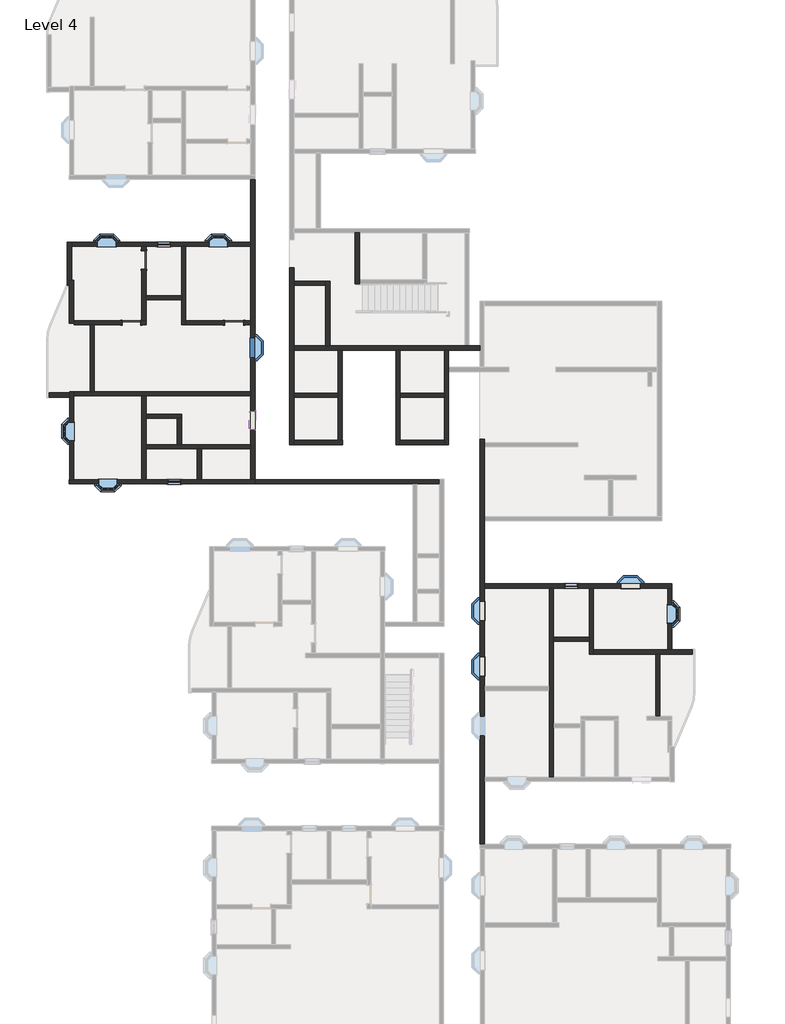
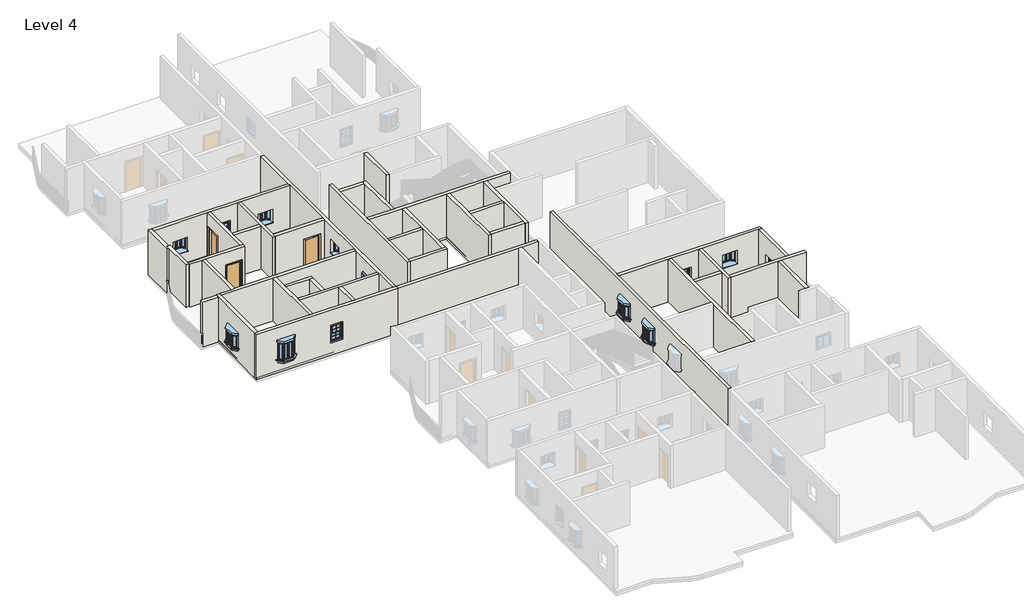
# One storey, part 3 of 14: 40 walls, 13 windows, 3 doors.
"""IFC4 building model written with IfcOpenShell, lengths in millimetres."""

from ifc_helpers import new_model, si_unit, frame, origin, place, context, project, spatial, polyline, outline, extrude, faceted_brep, transform, mapped, element, save
from components import door_54dd4da4, window_910x1210mm_154f9356, window_910x910mm_67ef725a, window_8debb0fa, windows_sgl_w_glazing_bars_910x910mm_256712d0

model = new_model("IFC4")

# Units and contexts
model_context = context("Model", 3, world=origin())
ifc_project = project(units=[si_unit("LENGTHUNIT", "METRE", prefix="MILLI")], contexts=[model_context])

# Site, building, storey
site = spatial("IfcSite", under=ifc_project)
building = spatial("IfcBuilding", under=site)
storey = spatial("IfcBuildingStorey", under=building, Name="Level 4", Elevation=9144.0)

# Doors
placement = place(None, origin())
door_shape = door_54dd4da4(model_context)
element("IfcDoor", 1, ObjectType="Single-Flush : 36\" x 84\"", at=placement, inside=storey, context=model_context, shape_type="MappedRepresentation", body=[
    mapped(door_shape, transform((-11210.3891351, 10605.7083494, 9144.0), x_axis=(1.0, 0.0, 0.0), y_axis=(0.0, 1.0, 0.0), z_axis=(0.0, 0.0, 1.0))),
])
element("IfcDoor", 2, ObjectType="Single-Flush : 36\" x 84\"", at=placement, inside=storey, context=model_context, shape_type="MappedRepresentation", body=[
    mapped(door_shape, transform((-15610.9391351, 13672.7583494, 9144.0), x_axis=(0.0, -1.0, 0.0), y_axis=(1.0, 0.0, 0.0), z_axis=(0.0, 0.0, 1.0))),
])
element("IfcDoor", 3, ObjectType="Single-Flush : 36\" x 84\"", at=placement, inside=storey, context=model_context, shape_type="MappedRepresentation", body=[
    mapped(door_shape, transform((-16220.5391351, 10605.7083494, 9144.0), x_axis=(1.0, 0.0, 0.0), y_axis=(0.0, 1.0, 0.0), z_axis=(0.0, 0.0, 1.0))),
])

# Walls
element("IfcWall", 4, ObjectType="4.5\" p", at=placement, inside=storey, context=model_context, shape_type="Brep", body=[
    faceted_brep([(-15509.3391351, 4456.3873146, 9144.0), (-13007.4391351, 4456.3873146, 9144.0), (-12804.2391351, 4456.3873146, 9144.0), (-10397.5891351, 4456.3873146, 9144.0), (-10397.5891351, 4456.3873146, 12192.0), (-12804.2391351, 4456.3873146, 12192.0), (-13007.4391351, 4456.3873146, 12192.0), (-15509.3391351, 4456.3873146, 12192.0), (-15509.3391351, 4659.5873146, 9144.0), (-15509.3391351, 4659.5873146, 12192.0), (-13985.3391351, 4659.5873146, 12192.0), (-13782.1391351, 4659.5873146, 12192.0), (-10397.5891351, 4659.5873146, 12192.0), (-10397.5891351, 4659.5873146, 9144.0), (-13782.1391351, 4659.5873146, 9144.0), (-13985.3391351, 4659.5873146, 9144.0)], [[[0, 1, 2, 3, 4, 5, 6, 7]], [[8, 9, 10, 11, 12, 13, 14, 15]], [[3, 2, 1, 0, 8, 15, 14, 13]], [[7, 6, 5, 4, 12, 11, 10, 9]], [[4, 3, 13, 12]], [[0, 7, 9, 8]]]),
])
element("IfcWall", 5, ObjectType="4.5\" p", at=placement, inside=storey, context=model_context, shape_type="SweptSolid", body=[
    extrude(outline(polyline([(-13007.4391351, 2953.9583494), (-13007.4391351, 4456.3873146), (-12804.2391351, 4456.3873146), (-12804.2391351, 2953.9583494), (-13007.4391351, 2953.9583494)])), frame((0.0, 0.0, 9144.0), z_axis=(0.0, 0.0, 1.0), x_axis=(1.0, 0.0, 0.0)), (0.0, 0.0, 1.0), 3048.0),
])
element("IfcWall", 6, ObjectType="4.5\" p", at=placement, inside=storey, context=model_context, shape_type="Brep", body=[
    faceted_brep([(-15509.3391351, 5953.2975261, 9144.0), (-13985.3391351, 5953.2975261, 9144.0), (-13782.1391351, 5953.2975261, 9144.0), (-13782.1391351, 5953.2975261, 12192.0), (-13985.3391351, 5953.2975261, 12192.0), (-15509.3391351, 5953.2975261, 12192.0), (-15509.3391351, 6156.4975261, 9144.0), (-15509.3391351, 6156.4975261, 12192.0), (-13782.1391351, 6156.4975261, 12192.0), (-13782.1391351, 6156.4975261, 9144.0)], [[[0, 1, 2, 3, 4, 5]], [[6, 7, 8, 9]], [[2, 1, 0, 6, 9]], [[5, 4, 3, 8, 7]], [[0, 5, 7, 6]], [[3, 2, 9, 8]]]),
])
element("IfcWall", 7, ObjectType="4.5\" p", at=placement, inside=storey, context=model_context, shape_type="SweptSolid", body=[
    extrude(outline(polyline([(-13985.3391351, 4659.5873146), (-13985.3391351, 5953.2975261), (-13782.1391351, 5953.2975261), (-13782.1391351, 4659.5873146), (-13985.3391351, 4659.5873146)])), frame((0.0, 0.0, 9144.0), z_axis=(0.0, 0.0, 1.0), x_axis=(1.0, 0.0, 0.0)), (0.0, 0.0, 1.0), 3048.0),
])
element("IfcWall", 8, ObjectType="4.5\" p", at=placement, inside=storey, context=model_context, shape_type="Brep", body=[
    faceted_brep([(-15712.5391351, 13215.5583494, 11277.6), (-15712.5391351, 13215.5583494, 9144.0), (-15712.5391351, 10707.3083494, 9144.0), (-15712.5391351, 10707.3083494, 12192.0), (-15712.5391351, 14333.1583494, 12192.0), (-15712.5391351, 14333.1583494, 9144.0), (-15712.5391351, 14129.9583494, 9144.0), (-15712.5391351, 14129.9583494, 11277.6), (-15509.3391351, 10707.3083494, 9144.0), (-15509.3391351, 11723.3083494, 9144.0), (-15509.3391351, 11926.5083494, 9144.0), (-15509.3391351, 13215.5583494, 9144.0), (-15509.3391351, 13215.5583494, 11277.6), (-15509.3391351, 14129.9583494, 11277.6), (-15509.3391351, 14129.9583494, 9144.0), (-15509.3391351, 14333.1583494, 9144.0), (-15509.3391351, 14333.1583494, 12192.0), (-15509.3391351, 11926.5083494, 12192.0), (-15509.3391351, 11723.3083494, 12192.0), (-15509.3391351, 10707.3083494, 12192.0)], [[[0, 1, 2, 3, 4, 5, 6, 7]], [[8, 9, 10, 11, 12, 13, 14, 15, 16, 17, 18, 19]], [[6, 5, 15, 14]], [[2, 1, 11, 10, 9, 8]], [[4, 3, 19, 18, 17, 16]], [[3, 2, 8, 19]], [[5, 4, 16, 15]], [[12, 11, 1, 0]], [[13, 12, 0, 7]], [[14, 13, 7, 6]]]),
])
element("IfcWall", 9, ObjectType="4.5\" p", at=placement, inside=storey, context=model_context, shape_type="Brep", body=[
    faceted_brep([(-13769.4391351, 14333.1583494, 9144.0), (-13769.4391351, 11926.5083494, 9144.0), (-13769.4391351, 11723.3083494, 9144.0), (-13769.4391351, 10504.1083494, 9144.0), (-13769.4391351, 10504.1083494, 12192.0), (-13769.4391351, 11723.3083494, 12192.0), (-13769.4391351, 11926.5083494, 12192.0), (-13769.4391351, 14333.1583494, 12192.0), (-13566.2391351, 14333.1583494, 9144.0), (-13566.2391351, 14333.1583494, 12192.0), (-13566.2391351, 10707.3083494, 12192.0), (-13566.2391351, 10504.1083494, 12192.0), (-13566.2391351, 10504.1083494, 9144.0), (-13566.2391351, 10707.3083494, 9144.0)], [[[0, 1, 2, 3, 4, 5, 6, 7]], [[8, 9, 10, 11, 12, 13]], [[3, 2, 1, 0, 8, 13, 12]], [[7, 6, 5, 4, 11, 10, 9]], [[0, 7, 9, 8]], [[4, 3, 12, 11]]]),
])
element("IfcWall", 10, ObjectType="4.5\" p", at=placement, inside=storey, context=model_context, shape_type="SweptSolid", body=[
    extrude(outline(polyline([(11277.6, -10753.1891351), (9144.0, -10753.1891351), (9144.0, -10397.5891351), (12192.0, -10397.5891351), (12192.0, -13566.2391351), (9144.0, -13566.2391351), (9144.0, -11667.5891351), (11277.6, -11667.5891351), (11277.6, -10753.1891351)])), frame((0.0, 10504.1083494, 0.0), z_axis=(0.0, 1.0, 0.0), x_axis=(0.0, 0.0, 1.0)), (0.0, 0.0, 1.0), 203.2),
])
element("IfcWall", 11, ObjectType="4.5\" p", at=placement, inside=storey, context=model_context, shape_type="SweptSolid", body=[
    extrude(outline(polyline([(-13769.4391351, 11723.3083494), (-15509.3391351, 11723.3083494), (-15509.3391351, 11926.5083494), (-13769.4391351, 11926.5083494), (-13769.4391351, 11723.3083494)])), frame((0.0, 0.0, 9144.0), z_axis=(0.0, 0.0, 1.0), x_axis=(1.0, 0.0, 0.0)), (0.0, 0.0, 1.0), 3048.0),
])
element("IfcWall", 12, ObjectType="4.5\" p", at=placement, inside=storey, context=model_context, shape_type="SweptSolid", body=[
    extrude(outline(polyline([(-6739.9891351, 12429.8715905), (-8289.3891351, 12429.8715905), (-8289.3891351, 12633.0715905), (-6739.9891351, 12633.0715905), (-6739.9891351, 12429.8715905)])), frame((0.0, 0.0, 9144.0), z_axis=(0.0, 0.0, 1.0), x_axis=(1.0, 0.0, 0.0)), (0.0, 0.0, 1.0), 3048.0),
])
element("IfcWall", 13, ObjectType="4.5\" p", at=placement, inside=storey, context=model_context, shape_type="SweptSolid", body=[
    extrude(outline(polyline([(-6130.3891351, 6970.2449943), (-8289.3891351, 6970.2449943), (-8289.3891351, 7173.4449943), (-6130.3891351, 7173.4449943), (-6130.3891351, 6970.2449943)])), frame((0.0, 0.0, 9144.0), z_axis=(0.0, 0.0, 1.0), x_axis=(1.0, 0.0, 0.0)), (0.0, 0.0, 1.0), 3048.0),
])
element("IfcWall", 14, ObjectType="4.5\" p", at=placement, inside=storey, context=model_context, shape_type="SweptSolid", body=[
    extrude(outline(polyline([(-948.7891351, 6970.2449943), (-3107.7891351, 6970.2449943), (-3107.7891351, 7173.4449943), (-948.7891351, 7173.4449943), (-948.7891351, 6970.2449943)])), frame((0.0, 0.0, 9144.0), z_axis=(0.0, 0.0, 1.0), x_axis=(1.0, 0.0, 0.0)), (0.0, 0.0, 1.0), 3048.0),
])
element("IfcWall", 15, ObjectType="4.5\" p", at=placement, inside=storey, context=model_context, shape_type="Brep", body=[
    faceted_brep([(-5298.5391351, 14988.9215905, 9144.0), (-5298.5391351, 12506.0715905, 9144.0), (-5298.5391351, 12506.0715905, 12192.0), (-5298.5391351, 14988.9215905, 12192.0), (-5095.3391351, 14988.9215905, 9144.0), (-5095.3391351, 14988.9215905, 12192.0), (-5095.3391351, 12709.2715905, 12192.0), (-5095.3391351, 12506.0715905, 12192.0), (-5095.3391351, 12506.0715905, 9144.0), (-5095.3391351, 12709.2715905, 9144.0)], [[[0, 1, 2, 3]], [[4, 5, 6, 7, 8, 9]], [[1, 0, 4, 9, 8]], [[3, 2, 7, 6, 5]], [[0, 3, 5, 4]], [[2, 1, 8, 7]]]),
])
element("IfcWall", 16, ObjectType="4.5\" p", at=placement, inside=storey, context=model_context, shape_type="SweptSolid", body=[
    extrude(outline(polyline([(-948.7891351, 4665.1949943), (-3107.7891351, 4665.1949943), (-3107.7891351, 4868.3949943), (-948.7891351, 4868.3949943), (-948.7891351, 4665.1949943)])), frame((0.0, 0.0, 9144.0), z_axis=(0.0, 0.0, 1.0), x_axis=(1.0, 0.0, 0.0)), (0.0, 0.0, 1.0), 3048.0),
])
element("IfcWall", 17, ObjectType="4.5\" p", at=placement, inside=storey, context=model_context, shape_type="Brep", body=[
    faceted_brep([(4184.4880523, -2336.4042694, 9144.0), (4184.4880523, -7130.6542694, 9144.0), (4184.4880523, -7333.8542694, 9144.0), (4184.4880523, -11556.6042694, 9144.0), (4184.4880523, -11556.6042694, 12192.0), (4184.4880523, -7333.8542694, 12192.0), (4184.4880523, -7130.6542694, 12192.0), (4184.4880523, -2336.4042694, 12192.0), (4387.6880523, -2336.4042694, 9144.0), (4387.6880523, -2336.4042694, 12192.0), (4387.6880523, -4736.7042694, 12192.0), (4387.6880523, -4939.9042694, 12192.0), (4387.6880523, -8959.4542694, 12192.0), (4387.6880523, -9162.6542694, 12192.0), (4387.6880523, -11556.6042694, 12192.0), (4387.6880523, -11556.6042694, 9144.0), (4387.6880523, -9162.6542694, 9144.0), (4387.6880523, -8959.4542694, 9144.0), (4387.6880523, -4939.9042694, 9144.0), (4387.6880523, -4736.7042694, 9144.0)], [[[0, 1, 2, 3, 4, 5, 6, 7]], [[8, 9, 10, 11, 12, 13, 14, 15, 16, 17, 18, 19]], [[3, 2, 1, 0, 8, 19, 18, 17, 16, 15]], [[7, 6, 5, 4, 14, 13, 12, 11, 10, 9]], [[4, 3, 15, 14]], [[0, 7, 9, 8]]]),
])
element("IfcWall", 18, ObjectType="4.5\" p", at=placement, inside=storey, context=model_context, shape_type="Brep", body=[
    faceted_brep([(803.8108649, 4915.2957306, 9144.0), (803.8108649, -14845.9042694, 9144.0), (803.8108649, -14845.9042694, 12192.0), (803.8108649, 4915.2957306, 12192.0), (803.8108649, -9516.0542694, 11254.0), (803.8108649, -9516.0542694, 10344.0), (803.8108649, -8606.0542694, 10344.0), (803.8108649, -8606.0542694, 11254.0), (803.8108649, -3909.0042694, 11254.0), (803.8108649, -3909.0042694, 10344.0), (803.8108649, -2999.0042694, 10344.0), (803.8108649, -2999.0042694, 11254.0), (803.8108649, -6620.4542694, 11254.0), (803.8108649, -6620.4542694, 10344.0), (803.8108649, -5710.4542694, 10344.0), (803.8108649, -5710.4542694, 11254.0), (1007.0108649, 4915.2957306, 9144.0), (1007.0108649, 4915.2957306, 12192.0), (1007.0108649, 4754.0949943, 12192.0), (1007.0108649, 4550.8949943, 12192.0), (1007.0108649, 1143.3957306, 12192.0), (1007.0108649, 940.1957306, 12192.0), (1007.0108649, -2133.2042694, 12192.0), (1007.0108649, -2336.4042694, 12192.0), (1007.0108649, -7130.6542694, 12192.0), (1007.0108649, -7333.8542694, 12192.0), (1007.0108649, -11556.6042694, 12192.0), (1007.0108649, -11759.8042694, 12192.0), (1007.0108649, -14845.9042694, 12192.0), (1007.0108649, -14845.9042694, 9144.0), (1007.0108649, -11759.8042694, 9144.0), (1007.0108649, -11556.6042694, 9144.0), (1007.0108649, -7333.8542694, 9144.0), (1007.0108649, -7130.6542694, 9144.0), (1007.0108649, -2336.4042694, 9144.0), (1007.0108649, -2133.2042694, 9144.0), (1007.0108649, 940.1957306, 9144.0), (1007.0108649, 1143.3957306, 9144.0), (1007.0108649, 4550.8949943, 9144.0), (1007.0108649, 4754.0949943, 9144.0), (1007.0108649, -9516.0542694, 11254.0), (1007.0108649, -8606.0542694, 11254.0), (1007.0108649, -8606.0542694, 10344.0), (1007.0108649, -9516.0542694, 10344.0), (1007.0108649, -3909.0042694, 11254.0), (1007.0108649, -2999.0042694, 11254.0), (1007.0108649, -2999.0042694, 10344.0), (1007.0108649, -3909.0042694, 10344.0), (1007.0108649, -6620.4542694, 11254.0), (1007.0108649, -5710.4542694, 11254.0), (1007.0108649, -5710.4542694, 10344.0), (1007.0108649, -6620.4542694, 10344.0)], [[[0, 1, 2, 3], [4, 5, 6, 7], [8, 9, 10, 11], [12, 13, 14, 15]], [[16, 17, 18, 19, 20, 21, 22, 23, 24, 25, 26, 27, 28, 29, 30, 31, 32, 33, 34, 35, 36, 37, 38, 39], [40, 41, 42, 43], [44, 45, 46, 47], [48, 49, 50, 51]], [[1, 0, 16, 39, 38, 37, 36, 35, 34, 33, 32, 31, 30, 29]], [[3, 2, 28, 27, 26, 25, 24, 23, 22, 21, 20, 19, 18, 17]], [[0, 3, 17, 16]], [[2, 1, 29, 28]], [[5, 4, 40, 43]], [[6, 5, 43, 42]], [[7, 6, 42, 41]], [[4, 7, 41, 40]], [[9, 8, 44, 47]], [[10, 9, 47, 46]], [[11, 10, 46, 45]], [[8, 11, 45, 44]], [[13, 12, 48, 51]], [[14, 13, 51, 50]], [[15, 14, 50, 49]], [[12, 15, 49, 48]]]),
])
element("IfcWall", 19, ObjectType="4.5\" p", at=placement, inside=storey, context=model_context, shape_type="SweptSolid", body=[
    extrude(outline(polyline([(6127.5880523, -4939.9042694), (4387.6880523, -4939.9042694), (4387.6880523, -4736.7042694), (6127.5880523, -4736.7042694), (6127.5880523, -4939.9042694)])), frame((0.0, 0.0, 9144.0), z_axis=(0.0, 0.0, 1.0), x_axis=(1.0, 0.0, 0.0)), (0.0, 0.0, 1.0), 3048.0),
])
element("IfcWall", 20, ObjectType="4.5\" p", at=placement, inside=storey, context=model_context, shape_type="Brep", body=[
    faceted_brep([(6127.5880523, -2336.4042694, 9144.0), (6127.5880523, -4736.7042694, 9144.0), (6127.5880523, -4939.9042694, 9144.0), (6127.5880523, -5555.8542694, 9144.0), (6127.5880523, -5555.8542694, 12192.0), (6127.5880523, -4939.9042694, 12192.0), (6127.5880523, -4736.7042694, 12192.0), (6127.5880523, -2336.4042694, 12192.0), (6330.7880523, -2336.4042694, 9144.0), (6330.7880523, -2336.4042694, 12192.0), (6330.7880523, -5352.6542694, 12192.0), (6330.7880523, -5555.8542694, 12192.0), (6330.7880523, -5555.8542694, 9144.0), (6330.7880523, -5352.6542694, 9144.0)], [[[0, 1, 2, 3, 4, 5, 6, 7]], [[8, 9, 10, 11, 12, 13]], [[3, 2, 1, 0, 8, 13, 12]], [[7, 6, 5, 4, 11, 10, 9]], [[0, 7, 9, 8]], [[4, 3, 12, 11]]]),
])
element("IfcWall", 21, ObjectType="4.5\" p", at=placement, inside=storey, context=model_context, shape_type="Brep", body=[
    faceted_brep([(6330.7880523, -5555.8542694, 9144.0), (9371.2322031, -5555.8542694, 9144.0), (9574.4322031, -5555.8542694, 9144.0), (11163.1380523, -5555.8542694, 9144.0), (11163.1380523, -5555.8542694, 12192.0), (9574.4322031, -5555.8542694, 12192.0), (9371.2322031, -5555.8542694, 12192.0), (6330.7880523, -5555.8542694, 12192.0), (6330.7880523, -5352.6542694, 9144.0), (6330.7880523, -5352.6542694, 12192.0), (9956.6380523, -5352.6542694, 12192.0), (10159.8380523, -5352.6542694, 12192.0), (11163.1380523, -5352.6542694, 12192.0), (11163.1380523, -5352.6542694, 9144.0), (10159.8380523, -5352.6542694, 9144.0), (9956.6380523, -5352.6542694, 9144.0)], [[[0, 1, 2, 3, 4, 5, 6, 7]], [[8, 9, 10, 11, 12, 13, 14, 15]], [[3, 2, 1, 0, 8, 15, 14, 13]], [[4, 3, 13, 12]], [[7, 6, 5, 4, 12, 11, 10, 9]], [[0, 7, 9, 8]]]),
])
element("IfcWall", 22, ObjectType="4.5\" p", at=placement, inside=storey, context=model_context, shape_type="SweptSolid", body=[
    extrude(outline(polyline([(9371.2322031, -8578.4542694), (9371.2322031, -5555.8542694), (9574.4322031, -5555.8542694), (9574.4322031, -8578.4542694), (9371.2322031, -8578.4542694)])), frame((0.0, 0.0, 9144.0), z_axis=(0.0, 0.0, 1.0), x_axis=(1.0, 0.0, 0.0)), (0.0, 0.0, 1.0), 3048.0),
])
element("IfcWall", 23, ObjectType="9\"", at=placement, inside=storey, context=model_context, shape_type="Brep", body=[
    faceted_brep([(-10181.6891351, 2953.9583494, 9144.0), (-10194.3891351, 2953.9583494, 9144.0), (-10397.5891351, 2953.9583494, 9144.0), (-12804.2391351, 2953.9583494, 9144.0), (-13007.4391351, 2953.9583494, 9144.0), (-15509.3391351, 2953.9583494, 9144.0), (-15712.5391351, 2953.9583494, 9144.0), (-19033.5891351, 2953.9583494, 9144.0), (-19236.7891351, 2953.9583494, 9144.0), (-19249.4891351, 2953.9583494, 9144.0), (-19249.4891351, 2953.9583494, 12192.0), (-19236.7891351, 2953.9583494, 12192.0), (-19033.5891351, 2953.9583494, 12192.0), (-15712.5391351, 2953.9583494, 12192.0), (-15509.3391351, 2953.9583494, 12192.0), (-13007.4391351, 2953.9583494, 12192.0), (-12804.2391351, 2953.9583494, 12192.0), (-10397.5891351, 2953.9583494, 12192.0), (-10194.3891351, 2953.9583494, 12192.0), (-10181.6891351, 2953.9583494, 12192.0), (-13794.8391351, 2953.9583494, 11125.2), (-14455.2391351, 2953.9583494, 11125.2), (-14455.2391351, 2953.9583494, 10058.4), (-13794.8391351, 2953.9583494, 10058.4), (-16918.0641351, 2953.9583494, 11268.4), (-17828.0641351, 2953.9583494, 11268.4), (-17828.0641351, 2953.9583494, 10058.4), (-16918.0641351, 2953.9583494, 10058.4), (-10181.6891351, 2750.7583494, 9144.0), (-10181.6891351, 2750.7583494, 12192.0), (-19249.4891351, 2750.7583494, 12192.0), (-19249.4891351, 2750.7583494, 9144.0), (-13794.8391351, 2750.7583494, 11125.2), (-13794.8391351, 2750.7583494, 10058.4), (-14455.2391351, 2750.7583494, 10058.4), (-14455.2391351, 2750.7583494, 11125.2), (-16918.0641351, 2750.7583494, 11268.4), (-16918.0641351, 2750.7583494, 10058.4), (-17828.0641351, 2750.7583494, 10058.4), (-17828.0641351, 2750.7583494, 11268.4)], [[[0, 1, 2, 3, 4, 5, 6, 7, 8, 9, 10, 11, 12, 13, 14, 15, 16, 17, 18, 19], [20, 21, 22, 23], [24, 25, 26, 27]], [[28, 29, 30, 31], [32, 33, 34, 35], [36, 37, 38, 39]], [[9, 8, 7, 6, 5, 4, 3, 2, 1, 0, 28, 31]], [[10, 9, 31, 30]], [[19, 18, 17, 16, 15, 14, 13, 12, 11, 10, 30, 29]], [[0, 19, 29, 28]], [[33, 32, 20, 23]], [[34, 33, 23, 22]], [[35, 34, 22, 21]], [[32, 35, 21, 20]], [[37, 36, 24, 27]], [[38, 37, 27, 26]], [[39, 38, 26, 25]], [[36, 39, 25, 24]]]),
])
element("IfcWall", 24, ObjectType="9\"", at=placement, inside=storey, context=model_context, shape_type="Brep", body=[
    faceted_brep([(-19033.5891351, 2953.9583494, 9144.0), (-19033.5891351, 7037.0083494, 9144.0), (-19033.5891351, 7240.2083494, 9144.0), (-19033.5891351, 7240.2083494, 12192.0), (-19033.5891351, 7037.0083494, 12192.0), (-19033.5891351, 2953.9583494, 12192.0), (-19033.5891351, 4854.8083494, 10968.4), (-19033.5891351, 5764.8083494, 10968.4), (-19033.5891351, 5764.8083494, 10058.4), (-19033.5891351, 4854.8083494, 10058.4), (-19236.7891351, 2953.9583494, 9144.0), (-19236.7891351, 2953.9583494, 12192.0), (-19236.7891351, 7240.2083494, 12192.0), (-19236.7891351, 7240.2083494, 9144.0), (-19236.7891351, 4854.8083494, 10968.4), (-19236.7891351, 4854.8083494, 10058.4), (-19236.7891351, 5764.8083494, 10058.4), (-19236.7891351, 5764.8083494, 10968.4)], [[[0, 1, 2, 3, 4, 5], [6, 7, 8, 9]], [[10, 11, 12, 13], [14, 15, 16, 17]], [[2, 1, 0, 10, 13]], [[5, 4, 3, 12, 11]], [[0, 5, 11, 10]], [[3, 2, 13, 12]], [[15, 14, 6, 9]], [[16, 15, 9, 8]], [[17, 16, 8, 7]], [[14, 17, 7, 6]]]),
])
element("IfcWall", 25, ObjectType="9\"", at=placement, inside=storey, context=model_context, shape_type="Brep", body=[
    faceted_brep([(-10194.3891351, 2953.9583494, 9144.0), (-10194.3891351, 17597.0583494, 9144.0), (-10194.3891351, 17597.0583494, 12192.0), (-10194.3891351, 2953.9583494, 12192.0), (-10194.3891351, 9841.5083494, 11254.0), (-10194.3891351, 9841.5083494, 10344.0), (-10194.3891351, 8931.5083494, 10344.0), (-10194.3891351, 8931.5083494, 11254.0), (-10194.3891351, 5393.297832, 11254.0), (-10194.3891351, 6303.297832, 11254.0), (-10194.3891351, 6303.297832, 10344.0), (-10194.3891351, 5393.297832, 10344.0), (-10397.5891351, 2953.9583494, 9144.0), (-10397.5891351, 2953.9583494, 12192.0), (-10397.5891351, 4456.3873146, 12192.0), (-10397.5891351, 4659.5873146, 12192.0), (-10397.5891351, 7037.0083494, 12192.0), (-10397.5891351, 7240.2083494, 12192.0), (-10397.5891351, 10504.1083494, 12192.0), (-10397.5891351, 10707.3083494, 12192.0), (-10397.5891351, 14333.1583494, 12192.0), (-10397.5891351, 14536.3583494, 12192.0), (-10397.5891351, 17597.0583494, 12192.0), (-10397.5891351, 17597.0583494, 9144.0), (-10397.5891351, 14536.3583494, 9144.0), (-10397.5891351, 14333.1583494, 9144.0), (-10397.5891351, 10707.3083494, 9144.0), (-10397.5891351, 10504.1083494, 9144.0), (-10397.5891351, 7240.2083494, 9144.0), (-10397.5891351, 7037.0083494, 9144.0), (-10397.5891351, 4659.5873146, 9144.0), (-10397.5891351, 4456.3873146, 9144.0), (-10397.5891351, 9841.5083494, 11254.0), (-10397.5891351, 8931.5083494, 11254.0), (-10397.5891351, 8931.5083494, 10344.0), (-10397.5891351, 9841.5083494, 10344.0), (-10397.5891351, 5393.297832, 11254.0), (-10397.5891351, 5393.297832, 10344.0), (-10397.5891351, 6303.297832, 10344.0), (-10397.5891351, 6303.297832, 11254.0)], [[[0, 1, 2, 3], [4, 5, 6, 7], [8, 9, 10, 11]], [[12, 13, 14, 15, 16, 17, 18, 19, 20, 21, 22, 23, 24, 25, 26, 27, 28, 29, 30, 31], [32, 33, 34, 35], [36, 37, 38, 39]], [[1, 0, 12, 31, 30, 29, 28, 27, 26, 25, 24, 23]], [[2, 1, 23, 22]], [[3, 2, 22, 21, 20, 19, 18, 17, 16, 15, 14, 13]], [[0, 3, 13, 12]], [[5, 4, 32, 35]], [[6, 5, 35, 34]], [[7, 6, 34, 33]], [[4, 7, 33, 32]], [[37, 36, 8, 11]], [[38, 37, 11, 10]], [[39, 38, 10, 9]], [[36, 39, 9, 8]]]),
])
element("IfcWall", 26, ObjectType="9\"", at=placement, inside=storey, context=model_context, shape_type="SweptSolid", body=[
    extrude(outline(polyline([(-19249.4891351, 6979.8583494), (-20240.0891351, 6979.8583494), (-20240.0891351, 7183.0583494), (-19249.4891351, 7183.0583494), (-19249.4891351, 6979.8583494)])), frame((0.0, 0.0, 9144.0), z_axis=(0.0, 0.0, 1.0), x_axis=(1.0, 0.0, 0.0)), (0.0, 0.0, 1.0), 3048.0),
])
element("IfcWall", 27, ObjectType="9\"", at=placement, inside=storey, context=model_context, shape_type="Brep", body=[
    faceted_brep([(-19147.8891351, 12435.1858981, 9144.0), (-19147.8891351, 14333.1583494, 9144.0), (-19147.8891351, 14536.3583494, 9144.0), (-19147.8891351, 14549.0583494, 9144.0), (-19147.8891351, 14549.0583494, 12192.0), (-19147.8891351, 14536.3583494, 12192.0), (-19147.8891351, 14333.1583494, 12192.0), (-19147.8891351, 12435.1858981, 12192.0), (-19351.0891351, 12435.1858981, 9144.0), (-19351.0891351, 12435.1858981, 12192.0), (-19351.0891351, 14549.0583494, 12192.0), (-19351.0891351, 14549.0583494, 9144.0)], [[[0, 1, 2, 3, 4, 5, 6, 7]], [[8, 9, 10, 11]], [[3, 2, 1, 0, 8, 11]], [[4, 3, 11, 10]], [[7, 6, 5, 4, 10, 9]], [[0, 7, 9, 8]]]),
])
element("IfcWall", 28, ObjectType="9\"", at=placement, inside=storey, context=model_context, shape_type="Brep", body=[
    faceted_brep([(-19147.8891351, 14333.1583494, 9144.0), (-15712.5391351, 14333.1583494, 9144.0), (-15509.3391351, 14333.1583494, 9144.0), (-13769.4391351, 14333.1583494, 9144.0), (-13566.2391351, 14333.1583494, 9144.0), (-10397.5891351, 14333.1583494, 9144.0), (-10397.5891351, 14333.1583494, 12192.0), (-13566.2391351, 14333.1583494, 12192.0), (-13769.4391351, 14333.1583494, 12192.0), (-15509.3391351, 14333.1583494, 12192.0), (-15712.5391351, 14333.1583494, 12192.0), (-19147.8891351, 14333.1583494, 12192.0), (-17885.2141351, 14333.1583494, 10968.4), (-16975.2141351, 14333.1583494, 10968.4), (-16975.2141351, 14333.1583494, 10058.4), (-17885.2141351, 14333.1583494, 10058.4), (-12436.9141351, 14333.1583494, 10968.4), (-11526.9141351, 14333.1583494, 10968.4), (-11526.9141351, 14333.1583494, 10058.4), (-12436.9141351, 14333.1583494, 10058.4), (-14309.1891351, 14333.1583494, 11125.2), (-14309.1891351, 14333.1583494, 10058.4), (-14969.5891351, 14333.1583494, 10058.4), (-14969.5891351, 14333.1583494, 11125.2), (-19147.8891351, 14536.3583494, 9144.0), (-19147.8891351, 14536.3583494, 12192.0), (-10397.5891351, 14536.3583494, 12192.0), (-10397.5891351, 14536.3583494, 9144.0), (-17885.2141351, 14536.3583494, 10968.4), (-17885.2141351, 14536.3583494, 10058.4), (-16975.2141351, 14536.3583494, 10058.4), (-16975.2141351, 14536.3583494, 10968.4), (-12436.9141351, 14536.3583494, 10968.4), (-12436.9141351, 14536.3583494, 10058.4), (-11526.9141351, 14536.3583494, 10058.4), (-11526.9141351, 14536.3583494, 10968.4), (-14309.1891351, 14536.3583494, 11125.2), (-14969.5891351, 14536.3583494, 11125.2), (-14969.5891351, 14536.3583494, 10058.4), (-14309.1891351, 14536.3583494, 10058.4)], [[[0, 1, 2, 3, 4, 5, 6, 7, 8, 9, 10, 11], [12, 13, 14, 15], [16, 17, 18, 19], [20, 21, 22, 23]], [[24, 25, 26, 27], [28, 29, 30, 31], [32, 33, 34, 35], [36, 37, 38, 39]], [[5, 4, 3, 2, 1, 0, 24, 27]], [[11, 10, 9, 8, 7, 6, 26, 25]], [[6, 5, 27, 26]], [[0, 11, 25, 24]], [[29, 28, 12, 15]], [[30, 29, 15, 14]], [[31, 30, 14, 13]], [[28, 31, 13, 12]], [[33, 32, 16, 19]], [[34, 33, 19, 18]], [[35, 34, 18, 17]], [[32, 35, 17, 16]], [[21, 20, 36, 39]], [[22, 21, 39, 38]], [[23, 22, 38, 37]], [[20, 23, 37, 36]]]),
])
element("IfcWall", 29, ObjectType="9\"", at=placement, inside=storey, context=model_context, shape_type="SweptSolid", body=[
    extrude(outline(polyline([(-19249.4891351, 10585.5474528), (-19249.4891351, 12672.4473407), (-19046.2891351, 12672.4473407), (-19046.2891351, 10585.5474528), (-19249.4891351, 10585.5474528)])), frame((0.0, 0.0, 9144.0), z_axis=(0.0, 0.0, 1.0), x_axis=(1.0, 0.0, 0.0)), (0.0, 0.0, 1.0), 3048.0),
])
element("IfcWall", 30, ObjectType="9\" w", at=placement, inside=storey, context=model_context, shape_type="Brep", body=[
    faceted_brep([(-1177.3891351, 2953.9583494, 9144.0), (-10181.6891351, 2953.9583494, 9144.0), (-10181.6891351, 2953.9583494, 12192.0), (-1177.3891351, 2953.9583494, 12192.0), (-1177.3891351, 2750.7583494, 9144.0), (-1177.3891351, 2750.7583494, 12192.0), (-2269.5891351, 2750.7583494, 12192.0), (-2472.7891351, 2750.7583494, 12192.0), (-10181.6891351, 2750.7583494, 12192.0), (-10181.6891351, 2750.7583494, 9144.0), (-2472.7891351, 2750.7583494, 9144.0), (-2269.5891351, 2750.7583494, 9144.0)], [[[0, 1, 2, 3]], [[4, 5, 6, 7, 8, 9, 10, 11]], [[1, 0, 4, 11, 10, 9]], [[2, 1, 9, 8]], [[3, 2, 8, 7, 6, 5]], [[0, 3, 5, 4]]]),
])
element("IfcWall", 31, ObjectType="9\" w", at=placement, inside=storey, context=model_context, shape_type="Brep", body=[
    faceted_brep([(-15763.3391351, 10504.1083494, 11277.6), (-15763.3391351, 10504.1083494, 9144.0), (-15509.3391351, 10504.1083494, 9144.0), (-15509.3391351, 10504.1083494, 12192.0), (-18042.9891351, 10504.1083494, 12192.0), (-18246.1891351, 10504.1083494, 12192.0), (-19027.2391351, 10504.1083494, 12192.0), (-19027.2391351, 10504.1083494, 9144.0), (-18246.1891351, 10504.1083494, 9144.0), (-18042.9891351, 10504.1083494, 9144.0), (-16677.7391351, 10504.1083494, 9144.0), (-16677.7391351, 10504.1083494, 11277.6), (-15509.3391351, 10707.3083494, 9144.0), (-15712.5391351, 10707.3083494, 9144.0), (-15763.3391351, 10707.3083494, 9144.0), (-15763.3391351, 10707.3083494, 11277.6), (-16677.7391351, 10707.3083494, 11277.6), (-16677.7391351, 10707.3083494, 9144.0), (-19027.2391351, 10707.3083494, 9144.0), (-19027.2391351, 10707.3083494, 12192.0), (-15712.5391351, 10707.3083494, 12192.0), (-15509.3391351, 10707.3083494, 12192.0)], [[[0, 1, 2, 3, 4, 5, 6, 7, 8, 9, 10, 11]], [[12, 13, 14, 15, 16, 17, 18, 19, 20, 21]], [[2, 1, 14, 13, 12]], [[10, 9, 8, 7, 18, 17]], [[6, 5, 4, 3, 21, 20, 19]], [[7, 6, 19, 18]], [[3, 2, 12, 21]], [[15, 14, 1, 0]], [[16, 15, 0, 11]], [[17, 16, 11, 10]]]),
])
element("IfcWall", 32, ObjectType="9\" w", at=placement, inside=storey, context=model_context, shape_type="SweptSolid", body=[
    extrude(outline(polyline([(-18246.1891351, 7240.2083494), (-18246.1891351, 10504.1083494), (-18042.9891351, 10504.1083494), (-18042.9891351, 7240.2083494), (-18246.1891351, 7240.2083494)])), frame((0.0, 0.0, 9144.0), z_axis=(0.0, 0.0, 1.0), x_axis=(1.0, 0.0, 0.0)), (0.0, 0.0, 1.0), 3048.0),
])
element("IfcWall", 33, ObjectType="9\" w", at=placement, inside=storey, context=model_context, shape_type="Brep", body=[
    faceted_brep([(-19033.5891351, 7037.0083494, 9144.0), (-15712.5391351, 7037.0083494, 9144.0), (-15509.3391351, 7037.0083494, 9144.0), (-10397.5891351, 7037.0083494, 9144.0), (-10397.5891351, 7037.0083494, 12192.0), (-15509.3391351, 7037.0083494, 12192.0), (-15712.5391351, 7037.0083494, 12192.0), (-19033.5891351, 7037.0083494, 12192.0), (-19033.5891351, 7240.2083494, 9144.0), (-19033.5891351, 7240.2083494, 12192.0), (-18246.1891351, 7240.2083494, 12192.0), (-18042.9891351, 7240.2083494, 12192.0), (-10397.5891351, 7240.2083494, 12192.0), (-10397.5891351, 7240.2083494, 9144.0), (-18042.9891351, 7240.2083494, 9144.0), (-18246.1891351, 7240.2083494, 9144.0)], [[[0, 1, 2, 3, 4, 5, 6, 7]], [[8, 9, 10, 11, 12, 13, 14, 15]], [[3, 2, 1, 0, 8, 15, 14, 13]], [[7, 6, 5, 4, 12, 11, 10, 9]], [[0, 7, 9, 8]], [[4, 3, 13, 12]]]),
])
element("IfcWall", 34, ObjectType="9\" w", at=placement, inside=storey, context=model_context, shape_type="Brep", body=[
    faceted_brep([(-15712.5391351, 7037.0083494, 9144.0), (-15712.5391351, 2953.9583494, 9144.0), (-15712.5391351, 2953.9583494, 12192.0), (-15712.5391351, 7037.0083494, 12192.0), (-15509.3391351, 7037.0083494, 9144.0), (-15509.3391351, 7037.0083494, 12192.0), (-15509.3391351, 6156.4975261, 12192.0), (-15509.3391351, 5953.2975261, 12192.0), (-15509.3391351, 4659.5873146, 12192.0), (-15509.3391351, 4456.3873146, 12192.0), (-15509.3391351, 2953.9583494, 12192.0), (-15509.3391351, 2953.9583494, 9144.0), (-15509.3391351, 4456.3873146, 9144.0), (-15509.3391351, 4659.5873146, 9144.0), (-15509.3391351, 5953.2975261, 9144.0), (-15509.3391351, 6156.4975261, 9144.0)], [[[0, 1, 2, 3]], [[4, 5, 6, 7, 8, 9, 10, 11, 12, 13, 14, 15]], [[1, 0, 4, 15, 14, 13, 12, 11]], [[3, 2, 10, 9, 8, 7, 6, 5]], [[2, 1, 11, 10]], [[0, 3, 5, 4]]]),
])
element("IfcWall", 35, ObjectType="9\" w", at=placement, inside=storey, context=model_context, shape_type="Brep", body=[
    faceted_brep([(-8492.5891351, 13295.1410318, 9144.0), (-8492.5891351, 4652.4949943, 9144.0), (-8492.5891351, 4652.4949943, 12192.0), (-8492.5891351, 13295.1410318, 12192.0), (-8289.3891351, 13295.1410318, 9144.0), (-8289.3891351, 13295.1410318, 12192.0), (-8289.3891351, 12633.0715905, 12192.0), (-8289.3891351, 12429.8715905, 12192.0), (-8289.3891351, 9478.4949943, 12192.0), (-8289.3891351, 9275.2949943, 12192.0), (-8289.3891351, 7173.4449943, 12192.0), (-8289.3891351, 6970.2449943, 12192.0), (-8289.3891351, 4868.3949943, 12192.0), (-8289.3891351, 4665.1949943, 12192.0), (-8289.3891351, 4652.4949943, 12192.0), (-8289.3891351, 4652.4949943, 9144.0), (-8289.3891351, 4665.1949943, 9144.0), (-8289.3891351, 4868.3949943, 9144.0), (-8289.3891351, 6970.2449943, 9144.0), (-8289.3891351, 7173.4449943, 9144.0), (-8289.3891351, 9275.2949943, 9144.0), (-8289.3891351, 9478.4949943, 9144.0), (-8289.3891351, 12429.8715905, 9144.0), (-8289.3891351, 12633.0715905, 9144.0)], [[[0, 1, 2, 3]], [[4, 5, 6, 7, 8, 9, 10, 11, 12, 13, 14, 15, 16, 17, 18, 19, 20, 21, 22, 23]], [[1, 0, 4, 23, 22, 21, 20, 19, 18, 17, 16, 15]], [[2, 1, 15, 14]], [[3, 2, 14, 13, 12, 11, 10, 9, 8, 7, 6, 5]], [[0, 3, 5, 4]]]),
])
element("IfcWall", 36, ObjectType="9\" w", at=placement, inside=storey, context=model_context, shape_type="Brep", body=[
    faceted_brep([(-8289.3891351, 4665.1949943, 9144.0), (-5914.4891351, 4665.1949943, 9144.0), (-5914.4891351, 4665.1949943, 12192.0), (-8289.3891351, 4665.1949943, 12192.0), (-8289.3891351, 4868.3949943, 9144.0), (-8289.3891351, 4868.3949943, 12192.0), (-6130.3891351, 4868.3949943, 12192.0), (-5927.1891351, 4868.3949943, 12192.0), (-5914.4891351, 4868.3949943, 12192.0), (-5914.4891351, 4868.3949943, 9144.0), (-5927.1891351, 4868.3949943, 9144.0), (-6130.3891351, 4868.3949943, 9144.0)], [[[0, 1, 2, 3]], [[4, 5, 6, 7, 8, 9, 10, 11]], [[1, 0, 4, 11, 10, 9]], [[2, 1, 9, 8]], [[3, 2, 8, 7, 6, 5]], [[0, 3, 5, 4]]]),
])
element("IfcWall", 37, ObjectType="9\" w", at=placement, inside=storey, context=model_context, shape_type="Brep", body=[
    faceted_brep([(-5927.1891351, 4868.3949943, 9144.0), (-5927.1891351, 9275.2949943, 9144.0), (-5927.1891351, 9275.2949943, 12192.0), (-5927.1891351, 4868.3949943, 12192.0), (-6130.3891351, 4868.3949943, 9144.0), (-6130.3891351, 4868.3949943, 12192.0), (-6130.3891351, 6970.2449943, 12192.0), (-6130.3891351, 7173.4449943, 12192.0), (-6130.3891351, 9275.2949943, 12192.0), (-6130.3891351, 9275.2949943, 9144.0), (-6130.3891351, 7173.4449943, 9144.0), (-6130.3891351, 6970.2449943, 9144.0)], [[[0, 1, 2, 3]], [[4, 5, 6, 7, 8, 9, 10, 11]], [[1, 0, 4, 11, 10, 9]], [[3, 2, 8, 7, 6, 5]], [[0, 3, 5, 4]], [[2, 1, 9, 8]]]),
])
element("IfcWall", 38, ObjectType="9\" w", at=placement, inside=storey, context=model_context, shape_type="Brep", body=[
    faceted_brep([(-8289.3891351, 9275.2949943, 9144.0), (-6130.3891351, 9275.2949943, 9144.0), (-5927.1891351, 9275.2949943, 9144.0), (-3310.9891351, 9275.2949943, 9144.0), (-3107.7891351, 9275.2949943, 9144.0), (-948.7891351, 9275.2949943, 9144.0), (-745.5891351, 9275.2949943, 9144.0), (793.5880523, 9275.2949943, 9144.0), (793.5880523, 9275.2949943, 12192.0), (-745.5891351, 9275.2949943, 12192.0), (-948.7891351, 9275.2949943, 12192.0), (-3107.7891351, 9275.2949943, 12192.0), (-3310.9891351, 9275.2949943, 12192.0), (-5927.1891351, 9275.2949943, 12192.0), (-6130.3891351, 9275.2949943, 12192.0), (-8289.3891351, 9275.2949943, 12192.0), (-8289.3891351, 9478.4949943, 9144.0), (-8289.3891351, 9478.4949943, 12192.0), (-6739.9891351, 9478.4949943, 12192.0), (-6536.7891351, 9478.4949943, 12192.0), (54.5108649, 9478.4949943, 12192.0), (257.7108649, 9478.4949943, 12192.0), (793.5880523, 9478.4949943, 12192.0), (793.5880523, 9478.4949943, 9144.0), (257.7108649, 9478.4949943, 9144.0), (54.5108649, 9478.4949943, 9144.0), (-6536.7891351, 9478.4949943, 9144.0), (-6739.9891351, 9478.4949943, 9144.0)], [[[0, 1, 2, 3, 4, 5, 6, 7, 8, 9, 10, 11, 12, 13, 14, 15]], [[16, 17, 18, 19, 20, 21, 22, 23, 24, 25, 26, 27]], [[7, 6, 5, 4, 3, 2, 1, 0, 16, 27, 26, 25, 24, 23]], [[15, 14, 13, 12, 11, 10, 9, 8, 22, 21, 20, 19, 18, 17]], [[0, 15, 17, 16]], [[8, 7, 23, 22]]]),
])
element("IfcWall", 39, ObjectType="9\" w", at=placement, inside=storey, context=model_context, shape_type="Brep", body=[
    faceted_brep([(-3310.9891351, 9275.2949943, 9144.0), (-3310.9891351, 4652.4949943, 9144.0), (-3310.9891351, 4652.4949943, 12192.0), (-3310.9891351, 9275.2949943, 12192.0), (-3107.7891351, 9275.2949943, 9144.0), (-3107.7891351, 9275.2949943, 12192.0), (-3107.7891351, 7173.4449943, 12192.0), (-3107.7891351, 6970.2449943, 12192.0), (-3107.7891351, 4868.3949943, 12192.0), (-3107.7891351, 4665.1949943, 12192.0), (-3107.7891351, 4652.4949943, 12192.0), (-3107.7891351, 4652.4949943, 9144.0), (-3107.7891351, 4665.1949943, 9144.0), (-3107.7891351, 4868.3949943, 9144.0), (-3107.7891351, 6970.2449943, 9144.0), (-3107.7891351, 7173.4449943, 9144.0)], [[[0, 1, 2, 3]], [[4, 5, 6, 7, 8, 9, 10, 11, 12, 13, 14, 15]], [[1, 0, 4, 15, 14, 13, 12, 11]], [[2, 1, 11, 10]], [[3, 2, 10, 9, 8, 7, 6, 5]], [[0, 3, 5, 4]]]),
])
element("IfcWall", 40, ObjectType="9\" w", at=placement, inside=storey, context=model_context, shape_type="Brep", body=[
    faceted_brep([(-745.5891351, 4652.4949943, 9144.0), (-745.5891351, 8223.6457306, 9144.0), (-745.5891351, 8426.8457306, 9144.0), (-745.5891351, 9275.2949943, 9144.0), (-745.5891351, 9275.2949943, 12192.0), (-745.5891351, 8426.8457306, 12192.0), (-745.5891351, 8223.6457306, 12192.0), (-745.5891351, 4652.4949943, 12192.0), (-948.7891351, 4652.4949943, 9144.0), (-948.7891351, 4652.4949943, 12192.0), (-948.7891351, 4665.1949943, 12192.0), (-948.7891351, 4868.3949943, 12192.0), (-948.7891351, 6970.2449943, 12192.0), (-948.7891351, 7173.4449943, 12192.0), (-948.7891351, 9275.2949943, 12192.0), (-948.7891351, 9275.2949943, 9144.0), (-948.7891351, 7173.4449943, 9144.0), (-948.7891351, 6970.2449943, 9144.0), (-948.7891351, 4868.3949943, 9144.0), (-948.7891351, 4665.1949943, 9144.0)], [[[0, 1, 2, 3, 4, 5, 6, 7]], [[8, 9, 10, 11, 12, 13, 14, 15, 16, 17, 18, 19]], [[3, 2, 1, 0, 8, 19, 18, 17, 16, 15]], [[7, 6, 5, 4, 14, 13, 12, 11, 10, 9]], [[0, 7, 9, 8]], [[4, 3, 15, 14]]]),
])
element("IfcWall", 41, ObjectType="9\" w", at=placement, inside=storey, context=model_context, shape_type="Brep", body=[
    faceted_brep([(-6536.7891351, 9478.4949943, 9144.0), (-6536.7891351, 12633.0715905, 9144.0), (-6536.7891351, 12633.0715905, 12192.0), (-6536.7891351, 9478.4949943, 12192.0), (-6739.9891351, 9478.4949943, 9144.0), (-6739.9891351, 9478.4949943, 12192.0), (-6739.9891351, 12429.8715905, 12192.0), (-6739.9891351, 12633.0715905, 12192.0), (-6739.9891351, 12633.0715905, 9144.0), (-6739.9891351, 12429.8715905, 9144.0)], [[[0, 1, 2, 3]], [[4, 5, 6, 7, 8, 9]], [[1, 0, 4, 9, 8]], [[3, 2, 7, 6, 5]], [[0, 3, 5, 4]], [[2, 1, 8, 7]]]),
])
element("IfcWall", 42, ObjectType="9\" w", at=placement, inside=storey, context=model_context, shape_type="Brep", body=[
    faceted_brep([(1007.0108649, -2336.4042694, 9144.0), (4184.4880523, -2336.4042694, 9144.0), (4387.6880523, -2336.4042694, 9144.0), (6127.5880523, -2336.4042694, 9144.0), (6330.7880523, -2336.4042694, 9144.0), (9956.6380523, -2336.4042694, 9144.0), (10159.8380523, -2336.4042694, 9144.0), (10172.5380523, -2336.4042694, 9144.0), (10172.5380523, -2336.4042694, 12192.0), (10159.8380523, -2336.4042694, 12192.0), (9956.6380523, -2336.4042694, 12192.0), (6330.7880523, -2336.4042694, 12192.0), (6127.5880523, -2336.4042694, 12192.0), (4387.6880523, -2336.4042694, 12192.0), (4184.4880523, -2336.4042694, 12192.0), (1007.0108649, -2336.4042694, 12192.0), (7688.7130523, -2336.4042694, 11254.0), (8598.7130523, -2336.4042694, 11254.0), (8598.7130523, -2336.4042694, 10344.0), (7688.7130523, -2336.4042694, 10344.0), (4927.4380523, -2336.4042694, 11125.2), (5587.8380523, -2336.4042694, 11125.2), (5587.8380523, -2336.4042694, 10058.4), (4927.4380523, -2336.4042694, 10058.4), (1007.0108649, -2133.2042694, 9144.0), (1007.0108649, -2133.2042694, 12192.0), (10172.5380523, -2133.2042694, 12192.0), (10172.5380523, -2133.2042694, 9144.0), (7688.7130523, -2133.2042694, 11254.0), (7688.7130523, -2133.2042694, 10344.0), (8598.7130523, -2133.2042694, 10344.0), (8598.7130523, -2133.2042694, 11254.0), (4927.4380523, -2133.2042694, 11125.2), (4927.4380523, -2133.2042694, 10058.4), (5587.8380523, -2133.2042694, 10058.4), (5587.8380523, -2133.2042694, 11125.2)], [[[0, 1, 2, 3, 4, 5, 6, 7, 8, 9, 10, 11, 12, 13, 14, 15], [16, 17, 18, 19], [20, 21, 22, 23]], [[24, 25, 26, 27], [28, 29, 30, 31], [32, 33, 34, 35]], [[7, 6, 5, 4, 3, 2, 1, 0, 24, 27]], [[8, 7, 27, 26]], [[15, 14, 13, 12, 11, 10, 9, 8, 26, 25]], [[0, 15, 25, 24]], [[29, 28, 16, 19]], [[30, 29, 19, 18]], [[31, 30, 18, 17]], [[28, 31, 17, 16]], [[33, 32, 20, 23]], [[34, 33, 23, 22]], [[35, 34, 22, 21]], [[32, 35, 21, 20]]]),
])
element("IfcWall", 43, ObjectType="9\" w", at=placement, inside=storey, context=model_context, shape_type="SweptSolid", body=[
    extrude(outline(polyline([(-2336.4042694, 9144.0), (-5352.6542694, 9144.0), (-5352.6542694, 12192.0), (-2336.4042694, 12192.0), (-2336.4042694, 9144.0)]), holes=[polyline([(-3151.4042694, 10968.4), (-4061.4042694, 10968.4), (-4061.4042694, 10058.4), (-3151.4042694, 10058.4), (-3151.4042694, 10968.4)])]), frame((9956.6380523, 0.0, 0.0), z_axis=(1.0, 0.0, 0.0), x_axis=(0.0, 1.0, 0.0)), (0.0, 0.0, 1.0), 203.2),
])

# Windows
window_910x1210mm_shape = window_910x1210mm_154f9356(model_context)
element("IfcWindow", 44, ObjectType="910x1210mm", at=placement, inside=storey, context=model_context, shape_type="MappedRepresentation", body=[
    mapped(window_910x1210mm_shape, transform((-17943.0641351, 2860.8149172, 9158.4), x_axis=(-1.0, 0.0, 0.0), y_axis=(0.0, -1.0, 0.0), z_axis=(0.0, 0.0, 1.0))),
])
window_910x910mm_shape = window_910x910mm_67ef725a(model_context)
element("IfcWindow", 45, ObjectType="910x910mm", at=placement, inside=storey, context=model_context, shape_type="MappedRepresentation", body=[
    mapped(window_910x910mm_shape, transform((8713.7130523, -2243.2608372, 9144.0), x_axis=(1.0, 0.0, 0.0), y_axis=(0.0, 1.0, 0.0), z_axis=(0.0, 0.0, 1.0))),
])
element("IfcWindow", 46, ObjectType="910x910mm", at=placement, inside=storey, context=model_context, shape_type="MappedRepresentation", body=[
    mapped(window_910x910mm_shape, transform((10049.7814845, -4176.4042694, 8858.4), x_axis=(0.0, -1.0, 0.0), y_axis=(1.0, 0.0, 0.0), z_axis=(0.0, 0.0, 1.0))),
])
element("IfcWindow", 47, ObjectType="910x910mm", at=placement, inside=storey, context=model_context, shape_type="MappedRepresentation", body=[
    mapped(window_910x910mm_shape, transform((-16860.2141351, 14426.3017816, 8858.4), x_axis=(1.0, 0.0, 0.0), y_axis=(0.0, 1.0, 0.0), z_axis=(0.0, 0.0, 1.0))),
])
element("IfcWindow", 48, ObjectType="910x910mm", at=placement, inside=storey, context=model_context, shape_type="MappedRepresentation", body=[
    mapped(window_910x910mm_shape, transform((-11411.9141351, 14426.3017816, 8858.4), x_axis=(1.0, 0.0, 0.0), y_axis=(0.0, 1.0, 0.0), z_axis=(0.0, 0.0, 1.0))),
])
element("IfcWindow", 49, ObjectType="910x910mm", at=placement, inside=storey, context=model_context, shape_type="MappedRepresentation", body=[
    mapped(window_910x910mm_shape, transform((-10304.445703, 8816.5083494, 9144.0), x_axis=(0.0, -1.0, 0.0), y_axis=(1.0, 0.0, 0.0), z_axis=(0.0, 0.0, 1.0))),
])
element("IfcWindow", 50, ObjectType="910x910mm", at=placement, inside=storey, context=model_context, shape_type="MappedRepresentation", body=[
    mapped(window_910x910mm_shape, transform((-19126.7325673, 5879.8083494, 8858.4), x_axis=(0.0, 1.0, 0.0), y_axis=(-1.0, 0.0, 0.0), z_axis=(0.0, 0.0, 1.0))),
])
element("IfcWindow", 51, ObjectType="910x910mm", at=placement, inside=storey, context=model_context, shape_type="MappedRepresentation", body=[
    mapped(window_910x910mm_shape, transform((913.8674327, -2884.0042694, 9144.0), x_axis=(0.0, 1.0, 0.0), y_axis=(-1.0, 0.0, 0.0), z_axis=(0.0, 0.0, 1.0))),
])
element("IfcWindow", 52, ObjectType="910x910mm", at=placement, inside=storey, context=model_context, shape_type="MappedRepresentation", body=[
    mapped(window_910x910mm_shape, transform((913.8674327, -5595.4542694, 9144.0), x_axis=(0.0, 1.0, 0.0), y_axis=(-1.0, 0.0, 0.0), z_axis=(0.0, 0.0, 1.0))),
])
window_shape = window_8debb0fa(model_context)
element("IfcWindow", 53, ObjectType="Window-Double-Hung : 26\" x 42\"", at=placement, inside=storey, context=model_context, shape_type="MappedRepresentation", body=[
    mapped(window_shape, transform((5257.6380523, -2234.8042694, 9144.0), x_axis=(1.0, 0.0, 0.0), y_axis=(0.0, 1.0, 0.0), z_axis=(0.0, 0.0, 1.0))),
])
element("IfcWindow", 54, ObjectType="Window-Double-Hung : 26\" x 42\"", at=placement, inside=storey, context=model_context, shape_type="MappedRepresentation", body=[
    mapped(window_shape, transform((-14639.3891351, 14434.7583494, 9144.0), x_axis=(-1.0, 0.0, 0.0), y_axis=(0.0, -1.0, 0.0), z_axis=(0.0, 0.0, 1.0))),
])
element("IfcWindow", 55, ObjectType="Window-Double-Hung : 26\" x 42\"", at=placement, inside=storey, context=model_context, shape_type="MappedRepresentation", body=[
    mapped(window_shape, transform((-14125.0391351, 2852.3583494, 9144.0), x_axis=(-1.0, 0.0, 0.0), y_axis=(0.0, -1.0, 0.0), z_axis=(0.0, 0.0, 1.0))),
])
windows_sgl_w_glazing_bars_910x910mm_shape = windows_sgl_w_glazing_bars_910x910mm_256712d0(model_context)
element("IfcWindow", 56, ObjectType="Windows_Sgl_w-Glazing_Bars : 910x910mm", at=placement, inside=storey, context=model_context, shape_type="MappedRepresentation", body=[
    mapped(windows_sgl_w_glazing_bars_910x910mm_shape, transform((-10287.5325673, 5848.297832, 9144.0), x_axis=(0.0, 1.0, 0.0), y_axis=(-1.0, 0.0, 0.0), z_axis=(0.0, 0.0, 1.0))),
])

save(model, "model.ifc")

# Revit data of these elements
# Type "Single-Flush : 36\" x 84\""
#   Type Mark = "1"
#   Construction Type Id = "MDOOR"
#   Assembly Code = "C1020"
#   Analytic Construction = "Metal"
#   Thickness = 0' - 2"
#   Heat Transfer Coefficient (U) = 0.651978 BTU/(h·ft²·°F)
#   Height = 7' - 0"
#   Trim Projection Ext = 0' - 1"
#   Trim Projection Int = 0' - 1"
#   Trim Width = 0' - 3"
#   Width = 3' - 0"
#   Define Thermal Properties by = 1
#   Define Thermal Properties by = 1
#   Door Material = Door - Panel
#   Frame Material = Door - Frame
#   Visual Light Transmittance = 0
#   Solar Heat Gain Coefficient = 0
#   Function = (empty or 0)
#   Wall Closure = (empty or 0)
# Type "4.5\" p"
#   Assembly Code = "B2010"
#   Layers, outside or top first: 0' - 8" no material (function 1)
# Type "9\""
#   Assembly Code = "B2010"
#   Layers, outside or top first: 0' - 8" no material (function 1)
# Type "9\" w"
#   Assembly Code = "B2010"
#   Layers, outside or top first: 0' - 8" no material (function 1)
# Type "910x1210mm"
#   Type Mark = "19"
#   Operation = "UserDefined"
#   Construction Type Id = "GSP4R"
#   Keynote = "L10"
#   Analytic Construction = "1/8 in Pilkington single glazing"
#   Wrap Layers (Ext) from Ext = 0' - 4.03543"
#   Wrap Layers (Int) from Ext = 0' - 6.98819"
#   Window Board Projection = 0' - 0.98425"
#   Window Board Extention = 0' - 0.98425"
#   Visual Light Transmittance = 0.9
#   Solar Heat Gain Coefficient = 0.78
#   Heat Transfer Coefficient (U) = 0.6496 BTU/(h·ft²·°F)
#   Glazing Thickness = 0' - 0.94488"
#   DONT CHANGE - Splay Width = 0' - 7.41997"
#   Rough Width = 2' - 11.82677"
#   Rough Height = 3' - 11.6378"
#   Roof Thickness = 0' - 4.92126"
#   Roof Overhang = 0' - 1.5748"
#   Plinth Thickness = 0' - 6.88976"
#   Height = 3' - 11.6378"
#   Width = 2' - 11.82677"
#   Frame Depth = 0' - 2.55906"
#   Default Head Height = 6' - 11.07087"
#   Cill Depth = 0' - 3.44488"
#   Cavity Closer Width = 0' - 1.9685"
#   Cavity Closer Offset from Ext = 0' - 4.03543"
#   Cavity Closer Depth = 0' - 3.34646"
#   Vis - Cavity Closers = yes
#   Define Thermal Properties by = 1
#   Material Trim = Window Frame
#   Material Glass = Glass
#   Material Frame = Window Frame
#   Manufacturer = ""
#   Wall Closure = (empty or 0)
# Type "910x910mm"
#   Type Mark = "18"
#   Operation = "UserDefined"
#   Construction Type Id = "GSP4R"
#   Keynote = "L10"
#   Analytic Construction = "1/8 in Pilkington single glazing"
#   Wrap Layers (Ext) from Ext = 0' - 4.03543"
#   Wrap Layers (Int) from Ext = 0' - 6.98819"
#   Window Board Projection = 0' - 0.98425"
#   Window Board Extention = 0' - 0.98425"
#   Visual Light Transmittance = 0.9
#   Solar Heat Gain Coefficient = 0.78
#   Heat Transfer Coefficient (U) = 0.6496 BTU/(h·ft²·°F)
#   Glazing Thickness = 0' - 0.94488"
#   DONT CHANGE - Splay Width = 0' - 7.41997"
#   Rough Width = 2' - 11.82677"
#   Rough Height = 2' - 11.82677"
#   Roof Thickness = 0' - 4.92126"
#   Roof Overhang = 0' - 1.5748"
#   Plinth Thickness = 0' - 6.88976"
#   Height = 2' - 11.82677"
#   Width = 2' - 11.82677"
#   Frame Depth = 0' - 2.55906"
#   Default Head Height = 6' - 11.07087"
#   Cill Depth = 0' - 3.44488"
#   Cavity Closer Width = 0' - 1.9685"
#   Cavity Closer Offset from Ext = 0' - 4.03543"
#   Cavity Closer Depth = 0' - 3.34646"
#   Vis - Cavity Closers = yes
#   Define Thermal Properties by = 1
#   Material Trim = Window Frame
#   Material Glass = Glass
#   Material Frame = Window Frame
#   Manufacturer = ""
#   Wall Closure = (empty or 0)
# Type "Window-Double-Hung : 26\" x 42\""
#   Type Mark = "11"
#   Fire Rating = "0.5h"
#   Construction Type Id = "DG-DR"
#   Assembly Code = "B2020100"
#   Analytic Construction = "Double glazing - domestic"
#   Wall Thickness [instance default] = 0' - 6"
#   Window Inset [instance default] = 0' - 0"
#   Visual Light Transmittance = 0.81
#   Thermal Resistance (R) = 1.8146 (h·ft²·°F)/BTU
#   Solar Heat Gain Coefficient = 0.76
#   Muntin Width = 1' - 8"
#   Muntin Height = 1' - 5 1/8"
#   Interior Wall Closure [instance default] = 0' - 1 1/2"
#   Rough Width = 2' - 2 1/2"
#   Rough Height = 3' - 6 1/2"
#   Frame Extension [instance default] = 0' - 1 1/4"
#   Exterior Wall Closure [instance default] = 0' - 0 1/2"
#   Extension Jamb [instance default] = 0' - 1 1/2"
#   Heat Transfer Coefficient (U) = 0.5511 BTU/(h·ft²·°F)
#   Height = 3' - 6"
#   Width = 2' - 2"
#   Define Thermal Properties by = 1
#   Top Muntin Visibility = yes
#   Indicator Visibility [instance default] = yes
#   Extension Jamb Visibility [instance default] = yes
#   Interior Trim Visibility [instance default] = yes
#   Exterior Trim Visibility [instance default] = yes
#   Define Thermal Properties by = 1
#   Bottom Muntin Visibility = yes
#   Muntin Pattern = Muntin Pattern_2x2 : Muntin Pattern_2x2
#   Interior Trim Material = Wood - Stained
#   Interior Trim = Trim-Window-Interior-Flat : Picture Frame
#   Exterior Trim Material = Clad - White
#   Exterior Trim = Trim-Window-Exterior-Flat : with Sill
#   Glass Panel Material = Glass
#   Exterior Frame Material = Clad - White
#   Interior Frame Material = Wood - Stained
#   Wall Closure = (empty or 0)
# Type "Windows_Sgl_w-Glazing_Bars : 910x910mm"
#   Type Mark = "24"
#   Operation = "SinglePanel"
#   Construction Type Id = "SGL"
#   Manufacturer = "Revit"
#   Keynote = "L10"
#   Analytic Construction = "Large single-glazed windows"
#   Wrap Layers (Ext) from Ext = 0' - 4.03543"
#   Wrap Layers (Int) from Ext = 0' - 6.98819"
#   Window Board Projection = 0' - 0.98425"
#   Window Board Extension = 0' - 0.98425"
#   Visual Light Transmittance = 0.9
#   Solar Heat Gain Coefficient = 0.86
#   Rough Width = 2' - 11.82677"
#   Rough Height = 2' - 11.82677"
#   Height = 2' - 11.82677"
#   Width = 2' - 11.82677"
#   Heat Transfer Coefficient (U) = 0.979472 BTU/(h·ft²·°F)
#   Glazing Thickness = 0' - 0.94488"
#   Glazing Bar Thickness = 0' - 0.7874"
#   FrameOffset - External = 0' - 3.14961"
#   Frame Depth = 0' - 2.55906"
#   Default Head Height = 6' - 11.07087"
#   Cill Depth = 0' - 3.44488"
#   Cavity Closer Width = 0' - 1.9685"
#   Cavity Closer Offset from Ext = 0' - 4.03543"
#   Cavity Closer Depth = 0' - 3.34646"
#   Vis - Glazing Bars = yes
#   Vis - Cavity Closers = yes
#   Define Thermal Properties by = 1
#   Material Trim = Window Frame
#   Material Glazing Bars = Window Frame
#   Material Glass = Glass
#   Material Frame = Window Frame
#   Wall Closure = (empty or 0)
# Elements 1, 2, 3 (IfcDoor, "Single-Flush : 36\" x 84\"")
#   Phase Created = New Construction
#   Materials on its faces: "Door - Frame", "Door - Panel"
# Elements 4, 5, 6, 7, 8, 9, 10, 11, 12, 13, 14, 15, 16, 17, 19, 20 (IfcWall, "4.5\" p")
#   Top Offset = 0' - 0"
#   Base Offset = 0' - 0"
#   wall height = 10' - 0"
#   Phase Created = New Construction
#   Base Constraint = Level 4
#   Top Constraint = Level 5
#   Materials on its faces: "Default Wall"
# Elements 18, 21 (IfcWall, "4.5\" p")
#   Top Offset = 0' - 0"
#   Base Offset = 0' - 0"
#   wall height = 10' - 0"
#   Phase Created = New Construction
#   Base Constraint = Level 4
#   Top Constraint = Level 5
#   Materials on its faces: "Default Wall", "Wood - Stained"
# Element 22 (IfcWall, "4.5\" p")
#   Top Offset = 0' - 0"
#   Base Offset = 0' - 0"
#   wall height = 10' - 0"
#   Phase Created = New Construction
#   Base Constraint = Level 4
#   Top Constraint = Level 5
#   Materials on its faces: "Default Wall", "Door - Frame"
# Element 23 (IfcWall, "9\"")
#   Top Offset = 0' - 0"
#   Base Offset = 0' - 0"
#   wall height = 10' - 0"
#   Phase Created = New Construction
#   Base Constraint = Level 4
#   Top Constraint = Level 5
#   Materials on its faces: "Default Wall", "Wood - Stained"
# Element 24 (IfcWall, "9\"")
#   Top Offset = 0' - 0"
#   Base Offset = 0' - 0"
#   wall height = 10' - 0"
#   Phase Created = New Construction
#   Base Constraint = Level 4
#   Top Constraint = Level 5
#   Materials on its faces: "Default Wall", "Cherry"
# Element 25 (IfcWall, "9\"")
#   Top Offset = 0' - 0"
#   Base Offset = 0' - 0"
#   wall height = 10' - 0"
#   Phase Created = New Construction
#   Base Constraint = Level 4
#   Top Constraint = Level 5
#   Materials on its faces: "Default Wall", "Parking Stripe"
